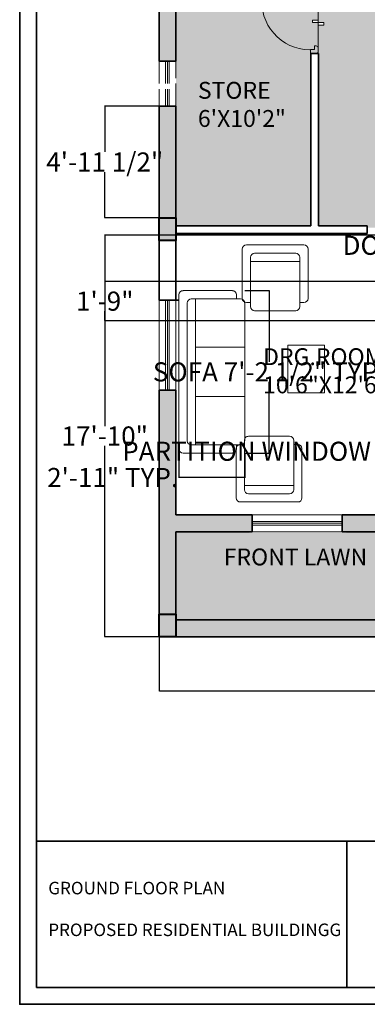
# Model space of a CAD drawing. Units: inches. Extents: x 1077 to 2505, y 1892 to 2728.
# Tile 19 of 26: x 1962 to 2147, y 1898 to 2423. Entities that reach past the tile are written whole.
import ezdxf

# ---------------------------------------------------------------- set-up
doc = ezdxf.new("R2010")
doc.units = ezdxf.units.IN
doc.linetypes.add('ACAD_ISO02W100', pattern=[15, 12, -3])
doc.layers.get('Defpoints').update_dxf_attribs({"color": 220, "linetype": 'ACAD_ISO02W100'})
for name, color, linetype, lineweight in [('00 FURNITURE', 15, 'Continuous', 15), ('A-ANNO-DIMS', 2, 'Continuous', 18), ('A-ANNO-TTLB', 7, 'Continuous', 35), ('A-AREA-IDEN', 7, 'Continuous', 18), ('A-COLS', 7, 'Continuous', 40), ('A-DOOR', 4, 'Continuous', 18), ('A-GLAZ-VENT', 6, 'ACAD_ISO02W100', 13), ('A-WALL-PATT', 7, 'Continuous', 9), ('A_FUR 1', 5, 'Continuous', 5), ('A_TEXT_SMALL', 18, 'Continuous', 13), ('WALL', 7, 'Continuous', 35), ('WINDOW', 160, 'Continuous', 13)]:
    doc.layers.add(name, color=color, linetype=linetype, lineweight=lineweight)
doc.layers.add('A-FLOR-PATT', color=254, linetype='Continuous', lineweight=9, true_color=0xd7ebd2)
doc.layers.add('L-PLNT-PATT', color=116, linetype='Continuous', lineweight=9, true_color=0x136734)
doc.styles.add('1-100DIM', font='txt', dxfattribs={"height": 0.3})
doc.styles.get("Standard").update_dxf_attribs({"font": 'arial.ttf'})
doc.dimstyles.get("Standard").update_dxf_attribs({"dimtxt": 10.18, "dimasz": 0.18, "dimexe": 0.18, "dimexo": 0.0625, "dimgap": 0.09, "dimtad": 0, "dimtih": 1, "dimtoh": 1, "dimdec": 0, "dimzin": 0, "dimdsep": 46, "dimlunit": 3, "dimtxsty": 'Standard', "dimcen": 0.09, "dimadec": 0, "dimazin": 0, "dimtfac": 1, "dimtdec": 0, "dimtofl": 0, "dimtmove": 0, "dimatfit": 3, "dimfxl": 1, "dimtolj": 1, "dimtzin": 0, "dimarcsym": 0})

# ---------------------------------------------------------------- blocks, each defined once
blk = doc.blocks.new('ESTSET')
at = {"layer": 'A_FUR 1'}
for p, q in [((-10.44, 4.1), (-10.44, 32.1)), ((-8.44, 4.1), (-8.44, 32.1)), ((-36.44, 6.1), (-36.44, 3.1)), ((-34.44, 6.1), (-36.44, 6.1)), ((-34.44, 4.1), (-34.44, 6.1)), ((-34.44, 4.1), (-34.44, 6.1)), ((-8.44, 4.1), (-8.44, 6.1)), ((-8.44, 6.1), (-6.44, 6.1)), ((-8.44, 4.1), (-8.44, 6.1)), ((-6.44, 6.1), (-6.44, 3.1)), ((-6.44, 2.1), (-36.44, 2.1)), ((-35.44, 2.1), (-33.44, 2.1)), ((-32.44, 4.1), (-34.44, 4.1)), ((-32.44, 4.1), (-34.44, 4.1)), ((-32.44, 3.1), (-32.44, 4.1)), ((-10.44, 3.1), (-10.44, 4.1)), ((-10.44, 4.1), (-8.44, 4.1)), ((-10.44, 4.1), (-8.44, 4.1)), ((-7.44, 2.1), (-9.44, 2.1))]:
    blk.add_line(p, q, dxfattribs=at)
for points in [[(-21.44, 2.1), (-18.67, 2.1), (-18.67, 5.1), (-20.06, 5.1)], [(-21.44, 2.1), (-21.44, -0.91), (-20.06, -0.91)], [(-20.06, 5.1), (-20.06, -0.91)]]:
    blk.add_lwpolyline(points, dxfattribs=at)
for centre, radius, start, end in [((-8.91, 6.46), 25.64, 88.9606, 185.2816), ((-35.44, 3.1), 1, 180, 270), ((-33.44, 3.1), 1, 270, 0), ((-9.44, 3.1), 1, 180, 270), ((-7.44, 3.1), 1, 270, 0)]:
    blk.add_arc(centre, radius, start, end, dxfattribs=at)
blk = doc.blocks.new('sofa 6')
for p, q in [((-1100, 167), (-1100, 834)), ((-1044, 890), (1044, 890)), ((1100, 834), (1100, 167)), ((-989, 56), (-989, 723)), ((-989, 667), (989, 667)), ((-933, 779), (933, 779)), ((-334, 667), (-334, 0)), ((334, 667), (334, 0)), ((989, 723), (989, 56)), ((-989, 111), (-1044, 111)), ((933, 0), (-933, 0)), ((1044, 111), (989, 111))]:
    blk.add_line(p, q)
for centre, start, end in [((-1044, 834), 90, 180), ((1044, 834), 0, 90), ((-933, 723), 90, 180), ((933, 723), 0, 90), ((-1044, 167), 180, 270), ((1044, 167), 270, 0), ((-933, 56), 180, 270), ((933, 56), 270, 0)]:
    blk.add_arc(centre, 55.6, start, end)
blk = doc.blocks.new('C1')
h = blk.add_hatch(color=256)
h.dxf.hatch_style = 1
h.paths.add_polyline_path([(1668.56, 2445.41), (1677.56, 2445.41), (1677.56, 2457.41), (1668.56, 2457.41)])
for p, q in [((1668.56, 2457.41), (1677.56, 2457.41)), ((1668.56, 2445.41), (1668.56, 2457.41)), ((1677.56, 2457.41), (1677.56, 2445.41)), ((1677.56, 2445.41), (1668.56, 2445.41))]:
    blk.add_line(p, q)
blk = doc.blocks.new('LOUNGE-ARMCHAIR')
for p, q in [((0, 6.57), (0, 32.85)), ((2.19, 35.04), (32.85, 35.04)), ((35.04, 32.85), (35.04, 6.57)), ((4.38, 2.19), (4.38, 28.47)), ((4.38, 26.28), (30.66, 26.28)), ((6.57, 30.66), (28.47, 30.66)), ((30.66, 28.47), (30.66, 2.19)), ((4.38, 4.38), (2.19, 4.38)), ((32.85, 4.38), (30.66, 4.38)), ((28.47, 0), (6.57, 0))]:
    blk.add_line(p, q)
for centre, start, end in [((2.19, 32.85), 90, 180), ((32.85, 32.85), 0, 90), ((6.57, 28.47), 90, 180), ((28.47, 28.47), 0, 90), ((2.19, 6.57), 180, 270), ((32.85, 6.57), 270, 0), ((6.57, 2.19), 180, 270), ((28.47, 2.19), 270, 0)]:
    blk.add_arc(centre, 2.19, start, end)
blk = doc.blocks.new('WINDOW-48-EXT')
for p, q in [((0, 48), (0, 0)), ((3.5, 48), (3.5, 0)), ((4.5, 48), (4.5, 0)), ((5.5, 48), (5.5, 0)), ((9, 0), (9, 48))]:
    blk.add_line(p, q)
blk = doc.blocks.new('VENT-24')
for p, q in [((3.5, 24), (3.5, 0)), ((4.5, 24), (4.5, 0)), ((5.5, 24), (5.5, 0))]:
    blk.add_line(p, q)
blk.add_lwpolyline([(0, 0), (9, 0), (9, 24), (0, 24)], close=True)
blk = doc.blocks.new('SHEET-FRAME-RESIDENTIAL')
for p, q in [((9, 87.01), (534.52, 87.01)), ((174.45, 87.01), (174.45, 9))]:
    blk.add_line(p, q)
for points in [[(0, 830.04), (543.52, 830.04), (543.52, 0), (0, 0)], [(9, 821.04), (534.52, 821.04), (534.52, 9), (9, 9)]]:
    blk.add_lwpolyline(points, close=True)
blk = doc.blocks.new('*D46')
at = {"layer": 'A-ANNO-DIMS', "color": 0, "lineweight": -2, "transparency": 16777216}
for p, q in [((2289.89, 2308.17), (2289.89, 2302.65)), ((2325.89, 2308.17), (2325.89, 2302.65)), ((2289.89, 2302.83), (2289.71, 2302.83)), ((2325.71, 2302.83), (2290.07, 2302.83))]:
    blk.add_line(p, q, dxfattribs=at)
at = {"layer": 'A-ANNO-DIMS', "color": 0, "transparency": 16777216}
for points in [[(2290.07, 2302.86), (2290.07, 2302.8), (2289.89, 2302.83)], [(2325.71, 2302.86), (2325.71, 2302.8), (2325.89, 2302.83)]]:
    blk.add_solid(points, dxfattribs=at)
at = {"layer": 'Defpoints', "color": 0, "transparency": 16777216}
for p in [(2289.89, 2308.23), (2325.89, 2308.23), (2289.89, 2302.83)]:
    blk.add_point(p, dxfattribs=at)
at = {"layer": 'A-ANNO-DIMS', "color": 0, "transparency": 16777216, "insert": (2209.47, 2302.83), "char_height": 10.18, "attachment_point": 5}
blk.add_mtext('\\A1;DOOR SWING 3\'-0" TYP.', dxfattribs=at)
blk = doc.blocks.new('*D50')
at = {"layer": 'A-ANNO-DIMS', "color": 0, "lineweight": -2, "transparency": 16777216}
for p, q in [((2219.31, 2200.18), (2219.31, 2192.86)), ((2267.31, 2200.18), (2267.31, 2192.86)), ((2219.31, 2193.04), (2219.13, 2193.04)), ((2267.13, 2193.04), (2219.49, 2193.04))]:
    blk.add_line(p, q, dxfattribs=at)
at = {"layer": 'A-ANNO-DIMS', "color": 0, "transparency": 16777216}
for points in [[(2219.49, 2193.07), (2219.49, 2193.01), (2219.31, 2193.04)], [(2267.13, 2193.07), (2267.13, 2193.01), (2267.31, 2193.04)]]:
    blk.add_solid(points, dxfattribs=at)
at = {"layer": 'Defpoints', "color": 0, "transparency": 16777216}
for p in [(2219.31, 2200.24), (2267.31, 2200.24), (2219.31, 2193.04)]:
    blk.add_point(p, dxfattribs=at)
at = {"layer": 'A-ANNO-DIMS', "color": 0, "transparency": 16777216, "insert": (2115.19, 2193.04), "char_height": 10.18, "attachment_point": 5}
blk.add_mtext('\\A1;PARTITION WINDOW 4\'-0" TYP.', dxfattribs=at)
blk = doc.blocks.new('*D54')
at = {"layer": 'A-ANNO-DIMS', "color": 0, "lineweight": -2, "transparency": 16777216}
for p, q in [((2081.59, 2278.66), (2094.7, 2278.66)), ((2094.52, 2278.48), (2094.52, 2240.71)), ((2094.52, 2192.23), (2094.52, 2230)), ((2081.59, 2192.05), (2094.7, 2192.05))]:
    blk.add_line(p, q, dxfattribs=at)
at = {"layer": 'A-ANNO-DIMS', "color": 0, "transparency": 16777216}
for points in [[(2094.49, 2278.48), (2094.55, 2278.48), (2094.52, 2278.66)], [(2094.49, 2192.23), (2094.55, 2192.23), (2094.52, 2192.05)]]:
    blk.add_solid(points, dxfattribs=at)
at = {"layer": 'Defpoints', "color": 0, "transparency": 16777216}
for p in [(2081.53, 2278.66), (2081.53, 2192.05), (2094.52, 2192.05)]:
    blk.add_point(p, dxfattribs=at)
at = {"layer": 'A-ANNO-DIMS', "color": 0, "transparency": 16777216, "insert": (2094.52, 2235.35), "char_height": 10.18, "attachment_point": 5}
blk.add_mtext('\\A1;SOFA 7\'-2 1/2" TYP.', dxfattribs=at)
blk = doc.blocks.new('*D55')
at = {"layer": 'A-ANNO-DIMS', "color": 0, "lineweight": -2, "transparency": 16777216}
for p, q in [((2046.49, 2191.98), (2046.49, 2178.87)), ((2081.53, 2191.98), (2081.53, 2178.87)), ((2046.49, 2179.05), (2046.31, 2179.05)), ((2081.35, 2179.05), (2046.67, 2179.05))]:
    blk.add_line(p, q, dxfattribs=at)
at = {"layer": 'A-ANNO-DIMS', "color": 0, "transparency": 16777216}
for points in [[(2046.67, 2179.08), (2046.67, 2179.02), (2046.49, 2179.05)], [(2081.35, 2179.08), (2081.35, 2179.02), (2081.53, 2179.05)]]:
    blk.add_solid(points, dxfattribs=at)
at = {"layer": 'Defpoints', "color": 0, "transparency": 16777216}
for p in [(2046.49, 2192.05), (2081.53, 2192.05), (2046.49, 2179.05)]:
    blk.add_point(p, dxfattribs=at)
at = {"layer": 'A-ANNO-DIMS', "color": 0, "transparency": 16777216, "insert": (2011.15, 2179.05), "char_height": 10.18, "attachment_point": 5}
blk.add_mtext('\\A1;2\'-11" TYP.', dxfattribs=at)
blk = doc.blocks.new('*D63')
at = {"layer": 'A-ANNO-DIMS', "color": 0, "lineweight": -2, "transparency": 16777216}
for p, q in [((2035.85, 2094.07), (2035.85, 2065.11)), ((2413.85, 2094.07), (2413.85, 2065.11)), ((2036.03, 2065.29), (2207.27, 2065.29)), ((2413.67, 2065.29), (2242.42, 2065.29))]:
    blk.add_line(p, q, dxfattribs=at)
at = {"layer": 'A-ANNO-DIMS', "color": 0, "transparency": 16777216}
for points in [[(2036.03, 2065.32), (2036.03, 2065.26), (2035.85, 2065.29)], [(2413.67, 2065.32), (2413.67, 2065.26), (2413.85, 2065.29)]]:
    blk.add_solid(points, dxfattribs=at)
at = {"layer": 'Defpoints', "color": 0, "transparency": 16777216}
for p in [(2035.85, 2094.14), (2413.85, 2094.14), (2413.85, 2065.29)]:
    blk.add_point(p, dxfattribs=at)
at = {"layer": 'A-ANNO-DIMS', "color": 0, "transparency": 16777216, "insert": (2224.85, 2065.29), "char_height": 10.18, "attachment_point": 5}
blk.add_mtext('\\A1;31\'-6"', dxfattribs=at)
blk = doc.blocks.new('*D68')
at = {"layer": 'A-ANNO-DIMS', "color": 0, "lineweight": -2, "transparency": 16777216}
for p, q in [((2289.82, 2308.23), (2006.75, 2308.23)), ((2006.93, 2308.05), (2006.93, 2206.47)), ((2006.93, 2094.32), (2006.93, 2195.9)), ((2289.78, 2094.14), (2006.75, 2094.14))]:
    blk.add_line(p, q, dxfattribs=at)
at = {"layer": 'A-ANNO-DIMS', "color": 0, "transparency": 16777216}
for points in [[(2006.9, 2308.05), (2006.96, 2308.05), (2006.93, 2308.23)], [(2006.9, 2094.32), (2006.96, 2094.32), (2006.93, 2094.14)]]:
    blk.add_solid(points, dxfattribs=at)
at = {"layer": 'Defpoints', "color": 0, "transparency": 16777216}
for p in [(2006.93, 2308.23), (2289.89, 2308.23), (2289.85, 2094.14)]:
    blk.add_point(p, dxfattribs=at)
at = {"layer": 'A-ANNO-DIMS', "color": 0, "transparency": 16777216, "insert": (2006.93, 2201.18), "char_height": 10.18, "attachment_point": 5}
blk.add_mtext('\\A1;17\'-10"', dxfattribs=at)
blk = doc.blocks.new('*D70')
at = {"layer": 'A-ANNO-DIMS', "color": 0, "lineweight": -2, "transparency": 16777216}
for p, q in [((2263.21, 2283.58), (2006.75, 2283.58)), ((2006.93, 2283.4), (2006.93, 2278.35)), ((2006.93, 2262.73), (2006.93, 2267.78)), ((2263.21, 2262.55), (2006.75, 2262.55))]:
    blk.add_line(p, q, dxfattribs=at)
at = {"layer": 'A-ANNO-DIMS', "color": 0, "transparency": 16777216}
for points in [[(2006.9, 2283.4), (2006.96, 2283.4), (2006.93, 2283.58)], [(2006.9, 2262.73), (2006.96, 2262.73), (2006.93, 2262.55)]]:
    blk.add_solid(points, dxfattribs=at)
at = {"layer": 'Defpoints', "color": 0, "transparency": 16777216}
for p in [(2006.93, 2283.58), (2263.27, 2283.58), (2263.27, 2262.55)]:
    blk.add_point(p, dxfattribs=at)
at = {"layer": 'A-ANNO-DIMS', "color": 0, "transparency": 16777216, "insert": (2006.93, 2273.06), "char_height": 10.18, "attachment_point": 5}
blk.add_mtext('\\A1;1\'-9"', dxfattribs=at)
blk = doc.blocks.new('*D75')
at = {"layer": 'A-ANNO-DIMS', "color": 0, "lineweight": -2, "transparency": 16777216}
for p, q in [((2035.79, 2377), (2006.75, 2377)), ((2006.93, 2376.82), (2006.93, 2352.59)), ((2006.93, 2317.65), (2006.93, 2341.88)), ((2035.8, 2317.47), (2006.75, 2317.47))]:
    blk.add_line(p, q, dxfattribs=at)
at = {"layer": 'A-ANNO-DIMS', "color": 0, "transparency": 16777216}
for points in [[(2006.9, 2376.82), (2006.96, 2376.82), (2006.93, 2377)], [(2006.9, 2317.65), (2006.96, 2317.65), (2006.93, 2317.47)]]:
    blk.add_solid(points, dxfattribs=at)
at = {"layer": 'Defpoints', "color": 0, "transparency": 16777216}
for p in [(2006.93, 2377), (2035.85, 2377), (2035.87, 2317.47)]:
    blk.add_point(p, dxfattribs=at)
at = {"layer": 'A-ANNO-DIMS', "color": 0, "transparency": 16777216, "insert": (2006.93, 2347.23), "char_height": 10.18, "attachment_point": 5}
blk.add_mtext('\\A1;4\'-11 1/2"', dxfattribs=at)

msp = doc.modelspace()

# ---------------------------------------------------------------- hatches: boundary and pattern name
at = {"layer": 'A-FLOR-PATT', "transparency": 33554559}
h = msp.add_hatch(color=256, dxfattribs=at)
h.dxf.hatch_style = 1
h.paths.add_polyline_path([(2252.85, 2583.14), (2232.15, 2583.14), (2208.15, 2583.17), (2208.15, 2583.14), (2186.85, 2583.14), (2186.85, 2486.14), (2186.85, 2475.14), (2182.85, 2475.14), (2182.85, 2521.11), (2164.84, 2521.11), (2164.84, 2583.14), (2126.63, 2583.14), (2078.63, 2583.13), (2078.63, 2583.14), (2044.85, 2583.14), (2044.85, 2439.14), (2146.85, 2439.14), (2146.85, 2435.14), (2120.85, 2435.14), (2044.85, 2435.14), (2044.85, 2401), (2044.85, 2401), (2044.85, 2377), (2044.85, 2377), (2044.85, 2313.14), (2116.85, 2313.14), (2116.85, 2405.14), (2120.85, 2405.14), (2120.85, 2313.14), (2146.85, 2313.14), (2146.85, 2312.21), (2182.85, 2312.21), (2182.85, 2313.14), (2186.85, 2313.14), (2186.85, 2312.21), (2222.85, 2312.21), (2222.85, 2313.14), (2289.85, 2313.14), (2289.85, 2094.14), (2404.85, 2094.14), (2404.85, 2146.06), (2368.85, 2146.06), (2368.85, 2273.14), (2332.85, 2273.14), (2332.85, 2309.14), (2325.85, 2309.14), (2325.85, 2313.14), (2404.85, 2313.14), (2404.85, 2354.2), (2404.85, 2402.2), (2404.85, 2435.14), (2292.85, 2435.14), (2292.85, 2439.14), (2333.66, 2439.14), (2333.66, 2457.16), (2404.85, 2457.16), (2404.85, 2583.14), (2356.85, 2583.14), (2356.85, 2592.14), (2404.85, 2592.14), (2404.85, 2648.14), (2375.5, 2648.14), (2375.5, 2648.03), (2351.47, 2648.03), (2351.47, 2648.14), (2326.85, 2648.14), (2326.85, 2583.14), (2256.85, 2583.14), (2256.85, 2435.14), (2182.85, 2435.14), (2182.85, 2439.14), (2186.85, 2439.14), (2252.85, 2439.14), (2252.85, 2486.14), (2216.85, 2486.14), (2216.85, 2490.14), (2252.85, 2490.14)])
h.paths.add_polyline_path([(2214.97, 2488.05), (2212.97, 2488.05), (2212.97, 2487.05, 0.414214), (2213.97, 2486.05), (2201.97, 2486.05), (2201.97, 2483.04), (2200.58, 2483.04), (2200.58, 2486.05), (2187.97, 2486.05, -0.414214), (2186.97, 2487.05), (2186.97, 2490.05), (2188.97, 2490.05), (2188.97, 2516.05, -0.446908)], flags=16)
h.paths.add_polyline_path([(2162.4, 2565.16), (2146.2, 2565.16), (2146.2, 2581.36), (2162.4, 2581.36)], flags=16)
h.paths.add_polyline_path([(2161.5, 2566.06), (2147.1, 2566.06), (2147.1, 2580.46), (2161.5, 2580.46)], flags=0)
h.paths.add_polyline_path([(2145.3, 2506.66, -0.414214), (2144.4, 2505.76), (2122.45, 2505.76), (2081.4, 2505.76, -0.414214), (2080.5, 2506.66), (2080.5, 2563.14), (2080.5, 2577.72), (2080.5, 2581.36), (2145.3, 2581.36), (2145.3, 2577.72), (2144.4, 2577.72, -0.414214), (2145.3, 2576.82)], flags=16)
h.paths.add_polyline_path([(2150.3, 2575.03, -1), (2158.24, 2575.03, -1)], flags=0)
h.paths.add_polyline_path([(2150.64, 2575.03, -1), (2157.89, 2575.03, -1)], flags=0)
h.paths.add_polyline_path([(2180.11, 2468.19), (2180.11, 2437.69), (2180.36, 2436.69), (2180.36, 2437.69), (2179.11, 2437.69), (2179.11, 2468.17, 0.404641), (2149.61, 2437.69), (2149.36, 2436.69, -0.414214), (2148.86, 2436.19), (2148.36, 2436.19), (2148.36, 2435.69, -0.414214), (2147.86, 2435.19), (2146.86, 2435.19), (2146.86, 2440.19), (2147.86, 2440.19, -0.414214), (2148.36, 2439.69), (2148.36, 2439.19), (2148.86, 2439.19, -0.414214), (2149.36, 2438.69), (2149.61, 2437.69, -0.414214)], flags=16)
h.paths.add_polyline_path([(2145.14, 2554.26, 0.292232), (2136.49, 2542.78, 0.052719), (2081.25, 2554.26), (2080.6, 2554.26), (2080.6, 2563.14), (2081.25, 2563.14), (2102.73, 2563.14, -0.117785), (2103.09, 2563.91, -0.059418), (2112.19, 2573, -0.379859), (2114.6, 2572.86, -0.02509), (2118.73, 2569.3, -0.025935), (2122.97, 2573, -0.379859), (2125.38, 2572.86, -0.061767), (2134.84, 2563.41, -0.069393), (2135.14, 2563.14), (2145.14, 2563.14)], flags=0)
h.paths.add_polyline_path([(2120.79, 2554.26), (2117.88, 2554.26, -0.015371), (2115.33, 2552.11, -0.429576), (2112.69, 2552.04, -0.016036), (2110.01, 2554.26), (2080.6, 2554.26), (2080.6, 2560.4), (2104.1, 2560.4, 0.055344), (2112.69, 2552.04, 0.331768), (2114.84, 2551.72, 0.027343), (2119.32, 2555.62, 0.00919)], flags=0)
h.paths.add_polyline_path([(2152.88, 2574.32), (2154.19, 2575.07), (2154.19, 2576.58, 0.399698), (2152.71, 2575.03, 0.119004)], flags=0)
h.paths.add_polyline_path([(2152.53, 2575.03, -1), (2156, 2575.03, -1)], flags=0)
h.paths.add_polyline_path([(2154.27, 2574.94), (2154.34, 2574.98), (2154.34, 2575.07), (2154.3, 2575.09), (2154.23, 2574.96)], flags=0)
h.paths.add_polyline_path([(2259.6, 2468.17, -0.414214), (2290.1, 2437.67), (2290.35, 2438.67), (2290.1, 2437.67, 0.404641), (2260.6, 2468.15), (2260.6, 2437.67), (2259.35, 2437.67), (2259.35, 2436.67, -0.414214), (2258.85, 2436.17), (2258.35, 2436.17), (2258.35, 2435.67, -0.414214), (2257.85, 2435.17), (2256.85, 2435.17), (2256.85, 2440.17), (2257.85, 2440.17, -0.414214), (2258.35, 2439.67), (2258.35, 2439.17), (2258.85, 2439.17, -0.414214), (2259.35, 2438.67)], flags=16)
h.paths.add_polyline_path([(2327.48, 2541.19, -0.414214), (2328.38, 2542.09), (2384.85, 2542.09), (2399.43, 2542.09), (2403.08, 2542.09), (2403.08, 2477.29), (2399.43, 2477.29), (2399.43, 2478.19, -0.414214), (2398.53, 2477.29), (2328.38, 2477.29, -0.414214), (2327.48, 2478.19), (2327.48, 2500.14)], flags=16)
h.paths.add_polyline_path([(2340.38, 2542.09, 0.253465), (2337.43, 2532.13, 0.2538), (2327.47, 2529.17)], flags=16)
h.paths.add_polyline_path([(2080.5, 2518.67, 0.253465), (2090.46, 2515.72, 0.2538), (2093.42, 2505.75)], flags=16)
h.paths.add_polyline_path([(2327.09, 2584.7), (2327.09, 2587.7), (2329.09, 2587.7), (2329.09, 2613.7, -0.01951), (2331.09, 2613.66), (2331.09, 2585.7), (2331.09, 2584.7, -0.414214), (2330.09, 2583.7), (2328.09, 2583.7, -0.414214)], flags=16)
h.paths.add_polyline_path([(2239.78, 2404.11), (2252.36, 2404.11), (2252.36, 2405.72), (2239.78, 2405.72)], flags=16)
h.paths.add_polyline_path([(2237.26, 2403.16), (2237.26, 2395.8), (2237.82, 2395.8), (2237.82, 2402.03, -0.41429), (2238.38, 2402.59), (2253.79, 2402.59, -0.414213), (2254.35, 2402.03), (2254.35, 2395.8), (2254.91, 2395.8), (2254.91, 2403.16)], flags=16)
h.paths.add_polyline_path([(2120.69, 2434.12), (2120.69, 2432.12, -0.414214), (2119.69, 2431.12), (2118.69, 2431.12), (2090.73, 2431.12, 0.400854), (2116.69, 2407.02), (2116.69, 2407.12), (2118.69, 2407.12, -0.446908), (2090.69, 2433.12), (2116.69, 2433.12), (2116.69, 2435.12), (2119.69, 2435.12, -0.414214)], flags=16)
h.paths.add_polyline_path([(2262.11, 2404.11), (2274.69, 2404.11), (2274.69, 2405.72), (2262.11, 2405.72)], flags=16)
h.paths.add_polyline_path([(2259.59, 2403.16), (2262.11, 2404.11), (2274.69, 2404.11), (2277.24, 2403.16)], flags=16)
h.paths.add_polyline_path([(2289.58, 2389.14), (2289.58, 2376.57), (2291.19, 2376.57), (2291.19, 2389.14)], flags=16)
h.paths.add_polyline_path([(2288.62, 2391.67), (2281.15, 2391.67), (2281.15, 2391.11), (2287.5, 2391.11, -0.41429), (2288.06, 2390.54), (2288.06, 2375.14, -0.414237), (2287.5, 2374.58), (2281.15, 2374.58), (2281.15, 2374.01), (2288.62, 2374.01)], flags=16)
h.paths.add_polyline_path([(2274.69, 2357.14), (2274.69, 2355.52), (2276.22, 2355.52, 0.414236), (2277.24, 2356.54), (2277.24, 2358.09)], flags=16)
h.paths.add_polyline_path([(2252.36, 2357.14), (2252.36, 2355.52), (2253.89, 2355.52, 0.414235), (2254.91, 2356.54), (2254.91, 2358.09)], flags=16)
h.paths.add_polyline_path([(2224.02, 2376.03), (2222.41, 2376.03), (2222.41, 2374.5, 0.414235), (2223.43, 2373.48), (2224.98, 2373.48)], flags=16)
h.paths.add_polyline_path([(2276.68, 2365.45), (2276.68, 2359.22, -0.41419), (2276.12, 2358.66), (2260.71, 2358.66, -0.414137), (2260.15, 2359.22), (2260.15, 2365.45), (2254.35, 2365.45), (2254.35, 2359.22, -0.414189), (2253.79, 2358.66), (2238.38, 2358.66, -0.414137), (2237.82, 2359.22), (2237.82, 2365.45)], flags=16)
h.paths.add_polyline_path([(2079.6, 2565.16), (2063.4, 2565.16), (2063.4, 2581.36), (2079.6, 2581.36)], flags=16)
h.paths.add_polyline_path([(2078.7, 2566.06), (2064.3, 2566.06), (2064.3, 2580.46), (2078.7, 2580.46)], flags=0)
h.paths.add_polyline_path([(2339.31, 2583.7), (2339.31, 2586.71), (2340.7, 2586.71), (2340.7, 2583.7), (2342.09, 2583.7), (2342.09, 2580.7), (2340.7, 2580.7), (2340.7, 2583.7)], flags=16)
h.paths.add_polyline_path([(2123.69, 2421.51), (2123.69, 2420.12), (2120.69, 2420.12), (2120.69, 2421.51), (2117.68, 2421.51), (2117.68, 2422.89), (2120.69, 2422.89), (2120.69, 2421.51)], flags=16)
h.paths.add_polyline_path([(2067.57, 2575.03, -1), (2075.51, 2575.03, -1)], flags=0)
h.paths.add_polyline_path([(2067.92, 2575.03, -1), (2075.17, 2575.03, -1)], flags=0)
h.paths.add_polyline_path([(2070.16, 2574.32), (2071.47, 2575.07), (2071.47, 2576.58, 0.399698), (2069.99, 2575.03, 0.119004)], flags=0)
h.paths.add_polyline_path([(2069.81, 2575.03, -1), (2073.28, 2575.03, -1)], flags=0)
h.paths.add_polyline_path([(2071.54, 2574.94), (2071.62, 2574.89), (2071.62, 2574.98)], flags=0)
h.paths.add_polyline_path([(2364.5, 2486.1, 0.052719), (2375.98, 2541.34), (2375.98, 2541.99), (2384.85, 2541.99), (2384.85, 2541.34), (2384.85, 2519.86, -0.117785), (2385.62, 2519.51, -0.059418), (2394.72, 2510.41, -0.379859), (2394.58, 2507.99, -0.02509), (2391.01, 2503.87, -0.025935), (2394.72, 2499.62, -0.379859), (2394.58, 2497.21, -0.061767), (2385.12, 2487.75, -0.069393), (2384.85, 2487.45), (2384.85, 2477.45), (2375.98, 2477.45, 0.292232)], flags=0)
h.paths.add_polyline_path([(2373.75, 2509.9, -0.016036), (2375.98, 2512.58), (2375.98, 2541.99), (2382.12, 2541.99), (2382.12, 2518.49, 0.055344), (2373.75, 2509.9, 0.331768), (2373.44, 2507.75, 0.027343), (2377.33, 2503.27, 0.00919), (2375.98, 2501.8), (2375.98, 2504.71, -0.015371), (2373.82, 2507.26, -0.429576)], flags=0)
h.paths.add_polyline_path([(2356.95, 2631.48, -0.171636), (2360.13, 2636.99), (2360.13, 2639.35), (2356, 2639.35, -0.414214), (2355.01, 2640.34), (2355.01, 2646.64, -0.414214), (2356, 2647.62), (2372.14, 2647.62, -0.414214), (2373.13, 2646.64), (2373.13, 2640.34, -0.414214), (2372.14, 2639.35), (2368.01, 2639.35), (2368.01, 2636.99, -0.171636), (2371.2, 2631.48, -0.258205), (2366.63, 2620.45), (2361.51, 2620.45, -0.258205)], flags=16)
h.paths.add_polyline_path([(2358.52, 2631.48, -0.171636), (2361.71, 2636.99), (2366.43, 2636.99, -0.171636), (2369.62, 2631.48, -0.210384), (2366.67, 2622), (2361.47, 2622, -0.210384)], flags=0)
h.paths.add_polyline_path([(2386.88, 2542.99), (2386.88, 2559.19), (2403.08, 2559.19), (2403.08, 2542.99)], flags=16)
h.paths.add_polyline_path([(2387.78, 2543.89), (2387.78, 2558.29), (2402.18, 2558.29), (2402.18, 2543.89)], flags=0)
h.paths.add_polyline_path([(2392.77, 2551.05, -1), (2400.71, 2551.05, -1)], flags=0)
h.paths.add_polyline_path([(2393.11, 2551.05, -1), (2400.37, 2551.05, -1)], flags=0)
h.paths.add_polyline_path([(2386.88, 2476.39), (2403.08, 2476.39), (2403.08, 2460.19), (2386.88, 2460.19)], flags=16)
h.paths.add_polyline_path([(2398.48, 2550.97), (2398.3, 2550.97, -0.544606), (2396.03, 2549.66), (2395.94, 2549.51, 0.547962)], flags=0)
h.paths.add_polyline_path([(2387.78, 2475.49), (2402.18, 2475.49), (2402.18, 2461.09), (2387.78, 2461.09)], flags=0)
h.paths.add_polyline_path([(2396.79, 2551.12), (2396.74, 2551.2), (2396.7, 2551.12)], flags=0)
h.paths.add_polyline_path([(2400.71, 2468.32, -1), (2392.77, 2468.32, -1)], flags=0)
h.paths.add_polyline_path([(2400.37, 2468.32, -1), (2393.11, 2468.32, -1)], flags=0)
h.paths.add_polyline_path([(2398.48, 2468.25), (2398.3, 2468.25, -0.544606), (2396.03, 2466.94), (2395.94, 2466.78, 0.547962)], flags=0)
h.paths.add_polyline_path([(2396.79, 2468.4), (2396.74, 2468.48), (2396.7, 2468.4)], flags=0)
h.paths.add_polyline_path([(2292.64, 2341.23, -0.414214), (2323.14, 2310.73), (2323.39, 2311.73), (2323.14, 2310.73, 0.404641), (2293.64, 2341.21), (2293.64, 2310.73), (2292.39, 2310.73), (2292.39, 2309.73, -0.414214), (2291.89, 2309.23), (2291.39, 2309.23), (2291.39, 2308.73, -0.414214), (2290.89, 2308.23), (2289.89, 2308.23), (2289.89, 2313.23), (2290.89, 2313.23, -0.414214), (2291.39, 2312.73), (2291.39, 2312.23), (2291.89, 2312.23, -0.414214), (2292.39, 2311.73)], flags=16)
h.paths.add_polyline_path([(2389.45, 2641.69), (2392.75, 2641.69), (2392.75, 2641.87), (2389.45, 2641.87)], flags=16)
edge = h.paths.add_edge_path(flags=16)
edge.add_arc((2393.3, 2638.65), 0.183, 270, 360)
edge.add_line((2393.49, 2638.65), (2393.49, 2645.8))
edge.add_line((2393.49, 2645.8), (2395.61, 2645.8))
edge.add_line((2395.61, 2645.8), (2395.61, 2647.8))
edge.add_line((2395.61, 2647.8), (2390.57, 2647.8))
edge.add_line((2390.57, 2647.8), (2390.57, 2645.8))
edge.add_line((2390.57, 2645.8), (2392.19, 2645.8))
edge.add_line((2392.19, 2645.8), (2392.19, 2644.98))
edge.add_line((2392.19, 2644.98), (2391.02, 2644.98))
edge.add_line((2391.02, 2644.98), (2391.02, 2645.8))
edge.add_line((2391.02, 2645.8), (2390.57, 2645.8))
edge.add_line((2390.57, 2645.8), (2390.57, 2647.8))
edge.add_line((2390.57, 2647.8), (2395.61, 2647.8))
edge.add_line((2395.61, 2647.8), (2395.61, 2647.32))
edge.add_line((2395.61, 2647.32), (2397.95, 2647.56))
edge.add_line((2397.95, 2647.56), (2397.95, 2647.8))
edge.add_line((2397.95, 2647.8), (2398.81, 2647.8))
edge.add_line((2398.81, 2647.8), (2398.81, 2647.23))
edge.add_line((2398.81, 2647.23), (2398.63, 2645.77))
edge.add_ellipse((2398.41, 2644.93), major_axis=(-1.08, 0), ratio=0.790849, start_angle=180, end_angle=255.2976, ccw=False)
edge.add_line((2399.49, 2644.93), (2399.49, 2644.36))
edge.add_ellipse((2398.41, 2644.36), major_axis=(-1.08, 0), ratio=0.790849, start_angle=0, end_angle=180, ccw=False)
edge.add_line((2397.32, 2644.36), (2397.33, 2644.85))
edge.add_ellipse((2398.41, 2644.93), major_axis=(-1.08, 0), ratio=0.790849, start_angle=284.7024, end_angle=364.0401, ccw=False)
edge.add_line((2398.1, 2645.73), (2398.1, 2647.23))
edge.add_line((2398.1, 2647.23), (2397.95, 2647.23))
edge.add_line((2397.95, 2647.23), (2395.61, 2646.99))
edge.add_line((2395.61, 2646.99), (2395.61, 2645.8))
edge.add_line((2395.61, 2645.8), (2393.49, 2645.8))
edge.add_line((2393.49, 2645.8), (2393.49, 2638.46))
edge.add_line((2393.49, 2638.46), (2393.3, 2638.46))
h.paths.add_polyline_path([(2353.64, 2256.32, -0.292371), (2356.22, 2253.81, -0.085148), (2358.52, 2214.83, -0.01331), (2357.59, 2104.48, -0.379287), (2354.54, 2101.26, -0.0502), (2298.86, 2101.26, -0.379287), (2295.81, 2104.48, -0.01331), (2294.88, 2214.83, -0.086132), (2297.28, 2254.24, -0.295116), (2299.9, 2256.76, -0.114238)], flags=16)
h.paths.add_polyline_path([(2352.48, 2211.82, -0.355389), (2354.02, 2208.08), (2350.26, 2195.63, -0.398275), (2346.44, 2193.45, 0.113332), (2306.96, 2193.45, -0.398275), (2303.14, 2195.63), (2299.38, 2208.08, -0.355394), (2300.92, 2211.82, -0.265725)], flags=0)
h.paths.add_polyline_path([(2297.68, 2201.7), (2303.26, 2187.65), (2303.26, 2166.61), (2298.16, 2163.24)], flags=0)
h.paths.add_polyline_path([(2355.78, 2201.7), (2355.31, 2163.24), (2350.2, 2166.61), (2350.2, 2187.65)], flags=0)
h.paths.add_polyline_path([(2303.26, 2164.35), (2303.26, 2143.1), (2298.44, 2128.54), (2298.19, 2161.01)], flags=0)
h.paths.add_polyline_path([(2350.2, 2164.35), (2355.28, 2161.01), (2355.03, 2128.54), (2350.2, 2143.1)], flags=0)
h.paths.add_polyline_path([(2347.2, 2136.38), (2351.71, 2113.65, -0.090102), (2301.76, 2113.63), (2306.27, 2136.37, 0.036636)], flags=0)
h.paths.add_polyline_path([(2304.86, 2165.32), (2354.76, 2165.32), (2354.76, 2183.87), (2304.86, 2183.87)], flags=8)
h.paths.add_polyline_path([(2053.76, 2360.82), (2103.97, 2360.82), (2103.97, 2394.41), (2053.76, 2394.41)], flags=24)
h.paths.add_polyline_path([(2153.41, 2366.23), (2211.12, 2366.23), (2211.12, 2399.82), (2153.41, 2399.82)], flags=24)
h.paths.add_polyline_path([(2258.04, 2477.83), (2327.95, 2477.83), (2327.95, 2511.42), (2258.04, 2511.42)], flags=24)
h.paths.add_polyline_path([(2182.1, 2454.46), (2252.27, 2454.46), (2252.27, 2473), (2182.1, 2473)], flags=24)
h.paths.add_polyline_path([(2192.4, 2537.41), (2246.99, 2537.41), (2246.99, 2571), (2192.4, 2571)], flags=24)
h.paths.add_polyline_path([(2083.07, 2465.98), (2152.99, 2465.98), (2152.99, 2499.56), (2083.07, 2499.56)], flags=24)
at = {"layer": 'A-WALL-PATT', "transparency": 33554585}
h = msp.add_hatch(color=256, dxfattribs=at)
h.dxf.hatch_style = 1
h.paths.add_polyline_path([(2044.85, 2429.98), (2035.85, 2429.98), (2035.85, 2401), (2044.85, 2401)])
h.paths.add_polyline_path([(2044.85, 2377), (2035.85, 2377), (2035.85, 2317.47), (2044.85, 2317.47)])
h.paths.add_polyline_path([(2085.45, 2159.14), (2044.85, 2159.14), (2044.85, 2225.64), (2035.85, 2225.64), (2035.85, 2106.16), (2044.85, 2106.16), (2044.85, 2150.14), (2085.45, 2150.14)])
h.paths.add_polyline_path([(2289.85, 2103.14), (2044.85, 2103.14), (2044.85, 2106.16), (2035.85, 2106.16), (2035.85, 2094.14), (2289.85, 2094.14)])
h.paths.add_polyline_path([(2413.85, 2354.2), (2404.85, 2354.2), (2404.85, 2354.2), (2404.85, 2313.14), (2325.85, 2313.14), (2325.85, 2309.14), (2404.85, 2309.14), (2404.85, 2094.14), (2413.85, 2094.14)])
h.paths.add_polyline_path([(2413.85, 2431.09), (2404.85, 2431.09), (2404.85, 2402.2), (2413.85, 2402.2)])
h.paths.add_polyline_path([(2404.85, 2439.14), (2292.85, 2439.14), (2292.85, 2435.14), (2404.85, 2435.14)])
h.paths.add_polyline_path([(2413.85, 2580.36), (2404.85, 2580.36), (2404.85, 2457.16), (2404.87, 2457.16), (2404.87, 2443.09), (2413.85, 2443.09)])
h.paths.add_polyline_path([(2413.85, 2645.09), (2404.85, 2645.09), (2404.85, 2592.36), (2413.85, 2592.36)])
h.paths.add_polyline_path([(2413.85, 2645.09), (2404.85, 2645.09), (2404.85, 2648.14), (2375.5, 2648.14), (2375.5, 2648.03), (2351.5, 2648.03), (2351.5, 2657.03), (2375.47, 2657.03), (2375.47, 2657.14), (2413.85, 2657.14)])
h.paths.add_polyline_path([(2351.47, 2657.14), (2326.92, 2657.14), (2326.92, 2648.14), (2351.47, 2648.14)])
h.paths.add_polyline_path([(2078.63, 2583.14), (2044.92, 2583.14), (2044.92, 2580.01), (2035.92, 2580.01), (2035.92, 2592.14), (2078.63, 2592.14)])
h.paths.add_polyline_path([(2180.39, 2592.14), (2126.63, 2592.14), (2126.63, 2583.14), (2180.39, 2583.14)])
h.paths.add_polyline_path([(2232.16, 2592.17), (2232.16, 2583.17), (2208.16, 2583.17), (2208.15, 2583.17), (2208.15, 2583.14), (2189.39, 2583.14), (2189.39, 2579.98), (2180.39, 2579.98), (2180.39, 2592.14), (2208.15, 2592.14), (2208.16, 2592.14), (2208.16, 2592.17)])
h.paths.add_polyline_path([(2250.27, 2592.14), (2232.16, 2592.14), (2232.16, 2583.14), (2250.27, 2583.14)], flags=17)
h.paths.add_polyline_path([(2326.85, 2648.14), (2326.92, 2657.14), (2317.85, 2657.14), (2317.85, 2592.14), (2250.27, 2592.14), (2250.27, 2583.14), (2252.85, 2583.14), (2252.85, 2490.14), (2216.85, 2490.14), (2216.85, 2486.14), (2252.85, 2486.14), (2252.85, 2439.14), (2186.85, 2439.14), (2182.85, 2439.14), (2182.85, 2435.14), (2256.85, 2435.14), (2256.85, 2583.14), (2326.85, 2583.14)])
h.paths.add_polyline_path([(2044.85, 2580.01), (2035.85, 2580.01), (2035.85, 2441.98), (2044.85, 2441.98)])
at = {"layer": 'A-WALL-PATT', "transparency": 33554559}
h = msp.add_hatch(color=256, dxfattribs=at)
h.dxf.hatch_style = 1
h.paths.add_polyline_path([(2146.85, 2439.14), (2044.78, 2439.14), (2044.78, 2435.14), (2120.85, 2435.14), (2146.85, 2435.14)])
h.paths.add_polyline_path([(2186.85, 2579.98), (2182.85, 2579.98), (2182.85, 2475.14), (2186.85, 2475.14), (2186.85, 2486.14)])
h.paths.add_polyline_path([(2404.83, 2592.14), (2356.85, 2592.14), (2356.85, 2587.7), (2357.09, 2587.7), (2357.09, 2584.7, -0.178139), (2356.85, 2584.05), (2356.85, 2583.14), (2404.83, 2583.14)])
h.paths.add_polyline_path([(2186.85, 2159.14), (2133.45, 2159.14), (2133.45, 2150.14), (2186.85, 2150.14)])
at = {"layer": 'L-PLNT-PATT', "transparency": 33554610}
h = msp.add_hatch(color=256, dxfattribs=at)
h.dxf.hatch_style = 1
h.paths.add_polyline_path([(2288.17, 2150.14), (2135.73, 2150.14), (2135.73, 2149.48), (2084.04, 2149.48), (2084.04, 2150.14), (2044.85, 2150.14), (2044.85, 2106.16), (2044.86, 2106.16), (2044.86, 2103.14), (2280.82, 2103.14), (2280.82, 2106.19), (2288.17, 2106.19)])
h.paths.add_polyline_path([(2067.09, 2127.13), (2154.7, 2127.13), (2154.7, 2145.68), (2067.09, 2145.68)], flags=24)

# ---------------------------------------------------------------- linework, layer by layer
at = {"layer": '00 FURNITURE'}
msp.add_lwpolyline([(2104.58, 2249.54), (2124.14, 2249.54), (2124.14, 2224.25), (2104.58, 2224.25)], close=True, dxfattribs=at)
at = {"layer": 'WALL'}
for p, q in [((2035.85, 2401), (2035.85, 2592.14)), ((2044.85, 2401), (2044.85, 2435.14)), ((2116.85, 2405.14), (2120.85, 2405.14)), ((2116.85, 2313.14), (2116.85, 2405.14)), ((2120.85, 2313.14), (2120.85, 2405.14)), ((2035.85, 2401), (2044.85, 2401)), ((2035.85, 2273.64), (2035.85, 2377)), ((2035.85, 2377), (2044.85, 2377)), ((2044.85, 2313.14), (2044.85, 2377)), ((2044.85, 2313.14), (2116.85, 2313.14)), ((2120.85, 2313.14), (2146.85, 2313.14)), ((2146.85, 2309.14), (2146.85, 2313.14)), ((2044.85, 2309.14), (2146.85, 2309.14)), ((2044.85, 2273.64), (2044.85, 2309.14)), ((2035.85, 2273.64), (2046.49, 2273.64)), ((2035.85, 2094.14), (2035.85, 2225.64)), ((2035.85, 2225.64), (2044.85, 2225.64)), ((2044.85, 2159.14), (2044.85, 2225.64)), ((2044.85, 2159.14), (2085.45, 2159.14)), ((2085.45, 2150.14), (2085.45, 2159.14)), ((2133.45, 2159.14), (2186.85, 2159.14)), ((2133.45, 2150.14), (2133.45, 2159.14)), ((2044.85, 2150.14), (2085.45, 2150.14)), ((2044.85, 2103.14), (2044.85, 2150.14)), ((2133.45, 2150.14), (2289.85, 2150.14)), ((2289.85, 2103.14), (2044.85, 2103.14)), ((2413.85, 2094.14), (2035.85, 2094.14))]:
    msp.add_line(p, q, dxfattribs=at)

# ---------------------------------------------------------------- block references
at = {"layer": '00 FURNITURE'}
msp.add_blockref('LOUNGE-ARMCHAIR', (2080.26, 2267.95), dxfattribs=at)
at = {"layer": '00 FURNITURE', "xscale": -0.0393700787401575, "yscale": 0.0393700787401575, "zscale": 0.0393700787401575, "rotation": 90}
msp.add_blockref('sofa 6', (2081.53, 2235.35), dxfattribs=at)
at = {"layer": '00 FURNITURE', "rotation": 180}
msp.add_blockref('LOUNGE-ARMCHAIR', (2112.05, 2201.04), dxfattribs=at)
at = {"layer": 'A-ANNO-TTLB'}
msp.add_blockref('SHEET-FRAME-RESIDENTIAL', (1961.57, 1898.25), dxfattribs=at)
at = {"layer": 'A-COLS'}
for p in [(367.31, -139.94), (367.3, -351.25)]:
    msp.add_blockref('C1', p, dxfattribs=at)
at = {"layer": 'A-DOOR', "rotation": 90.00000000000003}
msp.add_blockref('ESTSET', (2122.78, 2441.57), dxfattribs=at)
at = {"layer": 'A-GLAZ-VENT'}
msp.add_blockref('VENT-24', (2035.85, 2377), dxfattribs=at)
at = {"layer": 'WINDOW'}
for p, rotation in [((2044.85, 2273.65), 180), ((2133.45, 2150.14), 89.99999999999947)]:
    msp.add_blockref('WINDOW-48-EXT', p, dxfattribs=dict(at, rotation=rotation))

# ---------------------------------------------------------------- texts
at = {"layer": 'A-AREA-IDEN', "char_height": 9, "attachment_point": 1}
for s, insert in [('STORE\\P6\'X10\'2"', (2056.58, 2389.93)), ('\\pxi-3,l4,t4;DRG.ROOM\\P10\'6"X12\'6"', (2082.35, 2247.94)), ('FRONT LAWN', (2070.37, 2141.21))]:
    msp.add_mtext_dynamic_manual_height_columns(s, width=128.1076, gutter_width=12.5, heights=[0], dxfattribs=dict(at, insert=insert))
at = {"layer": 'A_TEXT_SMALL', "insert": (1976.81, 1963.54), "char_height": 6.6726, "attachment_point": 1, "style": '1-100DIM'}
msp.add_mtext_dynamic_manual_height_columns('{\\f@Malgun Gothic|b0|i0|c0|p34;GROUND FLOOR PLAN  \\P\\PPROPOSED RESIDENTIAL BUILDINGG}', width=159.0041, gutter_width=13.96, heights=[0], dxfattribs=at)

# ---------------------------------------------------------------- dimensions: what is measured, and where the dimension line sits
at = {"layer": 'A-ANNO-DIMS'}
for base, p1, p2, picture, middle in [((2006.93, 2377), (2035.87, 2317.47), (2035.85, 2377), '*D75', (2006.93, 2347.23)), ((2006.93, 2308.23), (2289.85, 2094.14), (2289.89, 2308.23), '*D68', (2006.93, 2201.18)), ((2006.93, 2283.58), (2263.27, 2262.55), (2263.27, 2283.58), '*D70', (2006.93, 2273.06))]:
    dim = msp.add_linear_dim(base=base, p1=p1, p2=p2, angle=90, dimstyle='Standard', override={"dimdec": 1, "dimlfac": 1, "dimrnd": 0, "dimzin": 1, "dimdsep": 46, "dimlunit": 4, "dimfrac": 2}, dxfattribs=at)
    dim.commit()
    dim.dimension.update_dxf_attribs({"geometry": picture, "text_midpoint": middle})
for base, p1, p2, angle, text, picture, middle in [((2289.89, 2302.83), (2325.89, 2308.23), (2289.89, 2308.23), 180, 'DOOR SWING <> TYP.', '*D46', (2209.47, 2302.83)), ((2094.52, 2192.05), (2081.53, 2278.66), (2081.53, 2192.05), 270, 'SOFA <> TYP.', '*D54', (2094.52, 2235.35)), ((2219.31, 2193.04), (2267.31, 2200.24), (2219.31, 2200.24), 180, 'PARTITION WINDOW <> TYP.', '*D50', (2115.19, 2193.04)), ((2046.49, 2179.05), (2081.53, 2192.05), (2046.49, 2192.05), 180, '<> TYP.', '*D55', (2011.15, 2179.05))]:
    dim = msp.add_linear_dim(base=base, p1=p1, p2=p2, angle=angle, text=text, dimstyle='Standard', override={"dimdec": 1, "dimlfac": 1, "dimrnd": 0, "dimzin": 1, "dimdsep": 46, "dimlunit": 4, "dimfrac": 2}, dxfattribs=at)
    dim.commit()
    dim.dimension.update_dxf_attribs({"geometry": picture, "text_midpoint": middle})
dim = msp.add_linear_dim(base=(2413.85, 2065.29), p1=(2035.85, 2094.14), p2=(2413.85, 2094.14), dimstyle='Standard', override={"dimdec": 1, "dimlfac": 1, "dimrnd": 0, "dimzin": 1, "dimdsep": 46, "dimlunit": 4, "dimfrac": 2}, dxfattribs=at)
dim.commit()
dim.dimension.update_dxf_attribs({"geometry": '*D63', "text_midpoint": (2224.85, 2065.29)})

doc.saveas('drawing.dxf')
